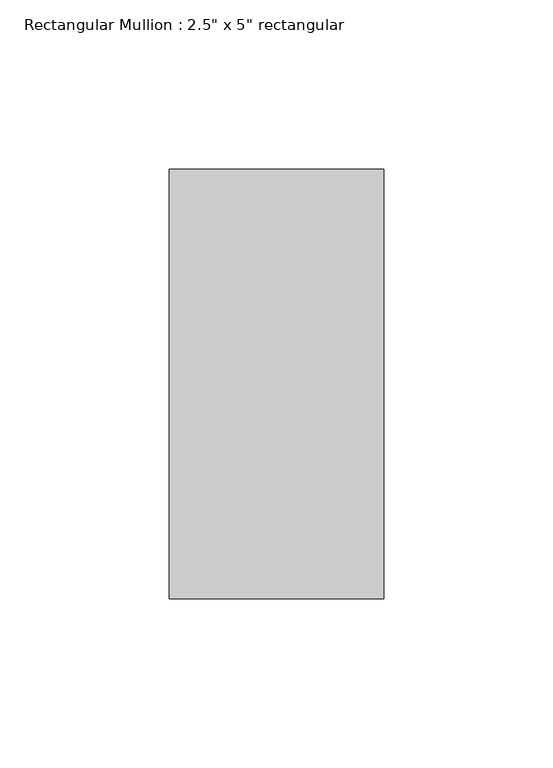
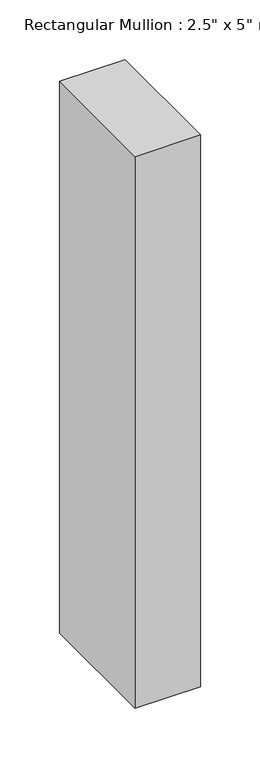
"""IFC4 building model written with IfcOpenShell, lengths in millimetres: member geometry."""

from ifc_helpers import new_model, si_unit, frame, origin, place, context, project, spatial, polyline, outline, extrude, source, transform, mapped, element, save


def member_6f432376(model_context):
    return source(origin(), model_context, "Body", "SweptSolid", [
        extrude(outline(polyline([(0.0, 63.5), (0.0, -63.5), (-63.5, -63.5), (-63.5, 63.5), (0.0, 63.5)])), frame((0.0, 0.0, -565.15), z_axis=(0.0, 0.0, 1.0), x_axis=(1.0, 0.0, 0.0)), (0.0, 0.0, 1.0), 565.15),
    ])


if __name__ == "__main__":
    model = new_model("IFC4")
    model_context = context("Model", 3, world=origin())
    ifc_project = project(units=[si_unit("LENGTHUNIT", "METRE", prefix="MILLI")], contexts=[model_context])
    site = spatial("IfcSite", under=ifc_project)
    building = spatial("IfcBuilding", under=site)
    placement = place(None, origin())
    member_shape = member_6f432376(model_context)
    element("IfcMember", 1, ObjectType="Rectangular Mullion : 2.5\" x 5\" rectangular", at=placement, inside=building, context=model_context, shape_type="MappedRepresentation", body=[
        mapped(member_shape, transform((0.0, 0.0, 0.0), x_axis=(1.0, 0.0, 0.0), y_axis=(0.0, 1.0, 0.0), z_axis=(0.0, 0.0, 1.0))),
    ])
    save(model, "model.ifc")

# Revit data of these elements
# Type "Rectangular Mullion : 2.5\" x 5\" rectangular"
#   built-in parameter 1007304 = 0.416667 (stored number, unit not read)
#   built-in parameter 1007301 = 0.104167 (stored number, unit not read)
#   built-in parameter 1007300 = 0.104167 (stored number, unit not read)
# Element 1 (IfcMember, "Rectangular Mullion : 2.5\" x 5\" rectangular")
#   Materials on its faces: "Aluminum"
# Materials
#   "Aluminum": class "Metal", colour RGB 247 247 247, transparency 0, Description = "Aluminum 6061", Cost = 0
